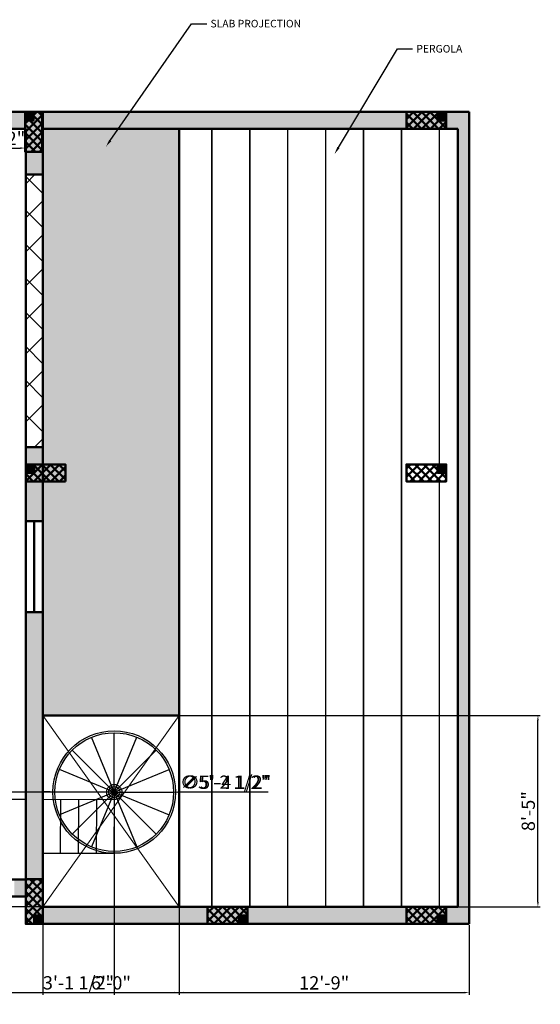
# Model space of a CAD drawing. Units: inches. Extents: x 1749 to 3550, y 1117 to 2383.
# Tile 12 of 15: x 3154 to 3428, y 1200 to 1720. Entities that reach past the tile are written whole.
import ezdxf
from ezdxf import colors
from ezdxf.entities.mleader import LeaderData, LeaderLine
from ezdxf.math import Vec2, Vec3

# ---------------------------------------------------------------- set-up
doc = ezdxf.new("R2010")
doc.units = ezdxf.units.IN
for name, color, linetype, lineweight in [('A-ANNO-DIMS', 2, 'Continuous', 18), ('A-ANNO-SYMB', 1, 'Continuous', 18), ('A-ANNO-TEXT', 3, 'Continuous', 18), ('A-COLS', 10, 'Continuous', 50), ('A-FLOR-STRS', 53, 'Continuous', 25), ('A-WALL', 7, 'Continuous', 50), ('A-WALL-PATT', 8, 'Continuous', 13)]:
    doc.layers.add(name, color=color, linetype=linetype, lineweight=lineweight)
doc.styles.get("Standard").update_dxf_attribs({"font": 'arial.ttf'})
doc.dimstyles.new('ISO-25', dxfattribs={"dimtxt": 7, "dimasz": 2.5, "dimexe": 1.25, "dimexo": 0.625, "dimtad": 1, "dimdec": 1, "dimlunit": 3, "dimtxsty": 'Standard', "dimcen": 2.5, "dimadec": 0, "dimazin": 0, "dimtfac": 1, "dimtdec": 1, "dimtmove": 0, "dimatfit": 3, "dimfxl": 1, "dimarcsym": 0})

# ---------------------------------------------------------------- blocks, each defined once
blk = doc.blocks.new('*D106')
at = {"layer": 'A-ANNO-DIMS', "color": 0, "lineweight": -2, "ltscale": 0.5, "transparency": 16777216}
for p, q in [((3122.34, 1661.76), (3122.34, 1651.06)), ((3156.55, 1661.76), (3156.55, 1651.06)), ((3124.84, 1652.31), (3154.05, 1652.31))]:
    blk.add_line(p, q, dxfattribs=at)
at = {"layer": 'A-ANNO-DIMS', "color": 0, "ltscale": 0.5, "transparency": 16777216}
for points in [[(3124.84, 1652.72), (3124.84, 1651.89), (3122.34, 1652.31)], [(3154.05, 1652.72), (3154.05, 1651.89), (3156.55, 1652.31)]]:
    blk.add_solid(points, dxfattribs=at)
at = {"layer": 'Defpoints', "color": 0, "ltscale": 0.5, "transparency": 16777216}
for p in [(3122.34, 1662.39), (3156.55, 1662.39), (3156.55, 1652.31)]:
    blk.add_point(p, dxfattribs=at)
at = {"layer": 'A-ANNO-DIMS', "color": 0, "ltscale": 0.5, "transparency": 16777216, "insert": (3139.44, 1656.51), "char_height": 7, "attachment_point": 5}
blk.add_mtext('2\'-10.2"', dxfattribs=at)
blk = doc.blocks.new('*D199')
at = {"layer": 'A-ANNO-DIMS', "color": 0, "lineweight": -2, "ltscale": 0.5, "transparency": 16777216}
for p, q in [((2730.84, 1242.26), (2730.84, 1205.39)), ((3390.84, 1242.26), (3390.84, 1205.39)), ((2733.34, 1206.64), (3388.34, 1206.64))]:
    blk.add_line(p, q, dxfattribs=at)
at = {"layer": 'A-ANNO-DIMS', "color": 0, "ltscale": 0.5, "transparency": 16777216}
for points in [[(2733.34, 1207.05), (2733.34, 1206.22), (2730.84, 1206.64)], [(3388.34, 1207.05), (3388.34, 1206.22), (3390.84, 1206.64)]]:
    blk.add_solid(points, dxfattribs=at)
at = {"layer": 'Defpoints', "color": 0, "ltscale": 0.5, "transparency": 16777216}
for p in [(2730.84, 1242.89), (3390.84, 1242.89), (3390.84, 1206.64)]:
    blk.add_point(p, dxfattribs=at)
at = {"layer": 'A-ANNO-DIMS', "color": 0, "ltscale": 0.5, "transparency": 16777216, "insert": (3060.84, 1210.84), "char_height": 7, "attachment_point": 5}
blk.add_mtext('55\'-0"', dxfattribs=at)
blk = doc.blocks.new('*D201')
at = {"layer": 'A-ANNO-DIMS', "color": 0, "lineweight": -2, "ltscale": 0.5, "transparency": 16777216}
for p, q in [((3237.84, 1251.26), (3237.84, 1205.39)), ((3165.84, 1242.26), (3165.84, 1205.39)), ((3168.34, 1206.64), (3235.34, 1206.64))]:
    blk.add_line(p, q, dxfattribs=at)
at = {"layer": 'A-ANNO-DIMS', "color": 0, "ltscale": 0.5, "transparency": 16777216}
for points in [[(3168.34, 1207.05), (3168.34, 1206.22), (3165.84, 1206.64)], [(3235.34, 1207.05), (3235.34, 1206.22), (3237.84, 1206.64)]]:
    blk.add_solid(points, dxfattribs=at)
at = {"layer": 'Defpoints', "color": 0, "ltscale": 0.5, "transparency": 16777216}
for p in [(3237.84, 1251.89), (3165.84, 1242.89), (3237.84, 1206.64)]:
    blk.add_point(p, dxfattribs=at)
at = {"layer": 'A-ANNO-DIMS', "color": 0, "ltscale": 0.5, "transparency": 16777216, "insert": (3201.84, 1210.84), "char_height": 7, "attachment_point": 5}
blk.add_mtext('6\'-0"', dxfattribs=at)
blk = doc.blocks.new('*D202')
at = {"layer": 'A-ANNO-DIMS', "color": 0, "lineweight": -2, "ltscale": 0.5, "transparency": 16777216}
for p, q in [((3237.84, 1251.26), (3237.84, 1205.39)), ((3390.84, 1242.26), (3390.84, 1205.39)), ((3240.34, 1206.64), (3388.34, 1206.64))]:
    blk.add_line(p, q, dxfattribs=at)
at = {"layer": 'A-ANNO-DIMS', "color": 0, "ltscale": 0.5, "transparency": 16777216}
for points in [[(3240.34, 1207.05), (3240.34, 1206.22), (3237.84, 1206.64)], [(3388.34, 1207.05), (3388.34, 1206.22), (3390.84, 1206.64)]]:
    blk.add_solid(points, dxfattribs=at)
at = {"layer": 'Defpoints', "color": 0, "ltscale": 0.5, "transparency": 16777216}
for p in [(3237.84, 1251.89), (3390.84, 1242.89), (3390.84, 1206.64)]:
    blk.add_point(p, dxfattribs=at)
at = {"layer": 'A-ANNO-DIMS', "color": 0, "ltscale": 0.5, "transparency": 16777216, "insert": (3314.34, 1210.84), "char_height": 7, "attachment_point": 5}
blk.add_mtext('12\'-9"', dxfattribs=at)
blk = doc.blocks.new('*D203')
at = {"layer": 'A-ANNO-DIMS', "color": 0, "lineweight": -2, "ltscale": 0.5, "transparency": 16777216}
for p, q in [((3203.57, 1311.82), (3203.57, 1205.39)), ((3165.84, 1308.09), (3165.84, 1205.39)), ((3168.34, 1206.64), (3201.07, 1206.64))]:
    blk.add_line(p, q, dxfattribs=at)
at = {"layer": 'A-ANNO-DIMS', "color": 0, "ltscale": 0.5, "transparency": 16777216}
for points in [[(3168.34, 1207.05), (3168.34, 1206.22), (3165.84, 1206.64)], [(3201.07, 1207.05), (3201.07, 1206.22), (3203.57, 1206.64)]]:
    blk.add_solid(points, dxfattribs=at)
at = {"layer": 'Defpoints', "color": 0, "ltscale": 0.5, "transparency": 16777216}
for p in [(3203.57, 1312.45), (3165.84, 1308.72), (3203.57, 1206.64)]:
    blk.add_point(p, dxfattribs=at)
at = {"layer": 'A-ANNO-DIMS', "color": 0, "ltscale": 0.5, "transparency": 16777216, "insert": (3184.7, 1210.88), "char_height": 7, "attachment_point": 5}
blk.add_mtext('3\'-1 1/2"', dxfattribs=at)
blk = doc.blocks.new('*D204')
at = {"layer": 'A-ANNO-DIMS', "color": 0, "lineweight": -2, "ltscale": 0.5, "transparency": 16777216}
for p, q in [((3202.94, 1312.45), (2693.34, 1312.45)), ((2694.59, 1254.39), (2694.59, 1309.95)), ((3165.21, 1251.89), (2693.34, 1251.89))]:
    blk.add_line(p, q, dxfattribs=at)
at = {"layer": 'A-ANNO-DIMS', "color": 0, "ltscale": 0.5, "transparency": 16777216}
for points in [[(2694.17, 1309.95), (2695, 1309.95), (2694.59, 1312.45)], [(2694.17, 1254.39), (2695, 1254.39), (2694.59, 1251.89)]]:
    blk.add_solid(points, dxfattribs=at)
at = {"layer": 'Defpoints', "color": 0, "ltscale": 0.5, "transparency": 16777216}
for p in [(2694.59, 1312.45), (3203.57, 1312.45), (3165.84, 1251.89)]:
    blk.add_point(p, dxfattribs=at)
at = {"layer": 'A-ANNO-DIMS', "color": 0, "ltscale": 0.5, "transparency": 16777216, "insert": (2690.34, 1282.17), "char_height": 7, "attachment_point": 5, "rotation": 90}
blk.add_mtext('5\'-0 1/2"', dxfattribs=at)
blk = doc.blocks.new('*D205')
at = {"layer": 'A-ANNO-DIMS', "color": 0, "lineweight": -2, "ltscale": 0.5, "transparency": 16777216}
for p, q in [((3238.46, 1352.89), (3428.34, 1352.89)), ((3427.09, 1254.39), (3427.09, 1350.39)), ((3238.46, 1251.89), (3428.34, 1251.89))]:
    blk.add_line(p, q, dxfattribs=at)
at = {"layer": 'A-ANNO-DIMS', "color": 0, "ltscale": 0.5, "transparency": 16777216}
for points in [[(3426.67, 1350.39), (3427.5, 1350.39), (3427.09, 1352.89)], [(3426.67, 1254.39), (3427.5, 1254.39), (3427.09, 1251.89)]]:
    blk.add_solid(points, dxfattribs=at)
at = {"layer": 'Defpoints', "color": 0, "ltscale": 0.5, "transparency": 16777216}
for p in [(3237.84, 1352.89), (3427.09, 1352.89), (3237.84, 1251.89)]:
    blk.add_point(p, dxfattribs=at)
at = {"layer": 'A-ANNO-DIMS', "color": 0, "ltscale": 0.5, "transparency": 16777216, "insert": (3422.89, 1302.39), "char_height": 7, "attachment_point": 5, "rotation": 90}
blk.add_mtext('8\'-5"', dxfattribs=at)
blk = doc.blocks.new('*D206')
at = {"layer": 'A-ANNO-DIMS', "color": 0, "lineweight": -2, "ltscale": 0.5, "transparency": 16777216}
for p, q in [((3168.73, 1312.5), (3166.23, 1312.5)), ((3171.23, 1312.49), (3235.9, 1312.4)), ((3284.69, 1312.33), (3238.4, 1312.4))]:
    blk.add_line(p, q, dxfattribs=at)
at = {"layer": 'A-ANNO-DIMS', "color": 0, "ltscale": 0.5, "transparency": 16777216}
for points in [[(3168.73, 1312.91), (3168.73, 1312.08), (3171.23, 1312.49)], [(3238.4, 1312.81), (3238.4, 1311.98), (3235.9, 1312.4)]]:
    blk.add_solid(points, dxfattribs=at)
at = {"layer": 'Defpoints', "color": 0, "ltscale": 0.5, "transparency": 16777216}
for p in [(3171.23, 1312.49), (3235.9, 1312.4)]:
    blk.add_point(p, dxfattribs=at)
at = {"layer": 'A-ANNO-DIMS', "color": 0, "ltscale": 0.5, "transparency": 16777216, "insert": (3262.8, 1316.76), "char_height": 7, "attachment_point": 5, "rotation": 359.9168}
blk.add_mtext('∅5\'-4 1/2"', dxfattribs=at)
blk = doc.blocks.new('*D207')
at = {"layer": 'A-ANNO-DIMS', "color": 0, "lineweight": -2, "ltscale": 0.5, "transparency": 16777216}
for p, q in [((3169.73, 1312.5), (3167.23, 1312.5)), ((3172.23, 1312.49), (3234.9, 1312.4)), ((3283.69, 1312.33), (3237.4, 1312.4))]:
    blk.add_line(p, q, dxfattribs=at)
at = {"layer": 'A-ANNO-DIMS', "color": 0, "ltscale": 0.5, "transparency": 16777216}
for points in [[(3169.73, 1312.91), (3169.73, 1312.08), (3172.23, 1312.49)], [(3237.4, 1312.81), (3237.4, 1311.98), (3234.9, 1312.4)]]:
    blk.add_solid(points, dxfattribs=at)
at = {"layer": 'Defpoints', "color": 0, "ltscale": 0.5, "transparency": 16777216}
for p in [(3172.23, 1312.49), (3234.9, 1312.4)]:
    blk.add_point(p, dxfattribs=at)
at = {"layer": 'A-ANNO-DIMS', "color": 0, "ltscale": 0.5, "transparency": 16777216, "insert": (3261.8, 1316.75), "char_height": 7, "attachment_point": 5, "rotation": 359.9141}
blk.add_mtext('∅5\'-2 1/2"', dxfattribs=at)

msp = doc.modelspace()

# ---------------------------------------------------------------- hatches: boundary and pattern name
at = {"layer": 'A-COLS', "ltscale": 10}
h = msp.add_hatch(color=256, dxfattribs=at)
h.dxf.hatch_style = 1
h.paths.add_polyline_path([(3156.55, 1671.39), (3156.55, 1666.89), (3161.05, 1666.89), (3161.05, 1671.39)])
h = msp.add_hatch(dxfattribs=at)
h.set_pattern_fill('ANSI37', color=256, angle=90)
h.set_pattern_definition([(135, (4539.2875, -0.8568), (-2.245064, -2.245064), []), (225, (4539.2875, -0.8568), (2.245064, -2.245064), [])])
h.paths.add_polyline_path([(3156.55, 1650.39), (3165.55, 1650.39), (3165.55, 1671.39), (3156.55, 1671.39)])
h = msp.add_hatch(dxfattribs=at)
h.set_pattern_fill('ANSI37', color=256, angle=180)
h.set_pattern_definition([(225, (5065.2954, 3029.4936), (2.245064, -2.245064), []), (315, (5065.2954, 3029.4936), (2.245064, 2.245064), [])])
h.paths.add_polyline_path([(3357.68, 1671.39), (3357.68, 1662.39), (3378.68, 1662.39), (3378.68, 1671.39)])
h = msp.add_hatch(color=256, dxfattribs=at)
h.dxf.hatch_style = 1
h.paths.add_polyline_path([(3378.68, 1671.39), (3374.18, 1671.39), (3374.18, 1666.89), (3378.68, 1666.89)])
h = msp.add_hatch(color=256, dxfattribs=at)
h.dxf.hatch_style = 1
h.paths.add_polyline_path([(3156.84, 1480.89), (3161.34, 1480.89), (3161.34, 1485.39), (3156.84, 1485.39)])
h = msp.add_hatch(dxfattribs=at)
h.set_pattern_fill('ANSI37', color=256, angle=180)
h.set_pattern_definition([(225, (4829.08, 2843.4936), (2.245064, -2.245064), []), (315, (4829.08, 2843.4936), (2.245064, 2.245064), [])])
h.paths.add_polyline_path([(3156.84, 1485.39), (3156.84, 1476.39), (3177.84, 1476.39), (3177.84, 1485.39)])
h = msp.add_hatch(dxfattribs=at)
h.set_pattern_fill('ANSI37', color=256, angle=360)
h.set_pattern_definition([(45, (1706.44, 96.9624), (-2.245064, 2.245064), []), (135, (1706.44, 96.9624), (-2.245064, -2.245064), [])])
h.paths.add_polyline_path([(3357.68, 1485.39), (3357.68, 1476.39), (3378.68, 1476.39), (3378.68, 1485.39)])
h = msp.add_hatch(color=256, dxfattribs=at)
h.dxf.hatch_style = 1
h.paths.add_polyline_path([(3378.68, 1485.39), (3374.18, 1485.39), (3374.18, 1480.89), (3378.68, 1480.89)])
h = msp.add_hatch(dxfattribs=at)
h.set_pattern_fill('ANSI37', color=256, angle=270)
h.set_pattern_definition([(315, (1770.86, 2915.132), (2.245064, 2.245064), []), (45, (1770.86, 2915.132), (-2.245064, 2.245064), [])])
h.paths.add_polyline_path([(3165.84, 1266.5), (3156.84, 1266.5), (3156.84, 1242.89), (3165.84, 1242.89)])
h = msp.add_hatch(color=256, dxfattribs=at)
h.dxf.hatch_style = 1
h.paths.add_polyline_path([(3165.84, 1242.89), (3165.84, 1247.39), (3161.34, 1247.39), (3161.34, 1242.89)])
h = msp.add_hatch(dxfattribs=at)
h.set_pattern_fill('ANSI37', color=256, angle=360)
h.set_pattern_definition([(45, (1601.591, -115.2184), (-2.245064, 2.245064), []), (135, (1601.591, -115.2184), (-2.245064, -2.245064), [])])
h.paths.add_polyline_path([(3273.84, 1242.89), (3273.84, 1251.89), (3252.84, 1251.89), (3252.84, 1242.89)])
h = msp.add_hatch(color=256, dxfattribs=at)
h.dxf.hatch_style = 1
h.paths.add_polyline_path([(3273.84, 1247.39), (3269.34, 1247.39), (3269.34, 1242.89), (3273.84, 1242.89)])
h = msp.add_hatch(dxfattribs=at)
h.set_pattern_fill('ANSI37', color=256, angle=360)
h.set_pattern_definition([(45, (1706.44, -115.2184), (-2.245064, 2.245064), []), (135, (1706.44, -115.2184), (-2.245064, -2.245064), [])])
h.paths.add_polyline_path([(3378.68, 1242.89), (3378.68, 1251.89), (3357.68, 1251.89), (3357.68, 1242.89)])
h = msp.add_hatch(color=256, dxfattribs=at)
h.dxf.hatch_style = 1
h.paths.add_polyline_path([(3378.68, 1247.39), (3374.18, 1247.39), (3374.18, 1242.89), (3378.68, 1242.89)])
at = {"layer": 'A-WALL-PATT', "ltscale": 0.5}
h = msp.add_hatch(color=256, dxfattribs=at)
h.dxf.hatch_style = 1
h.paths.add_polyline_path([(3156.84, 1662.39), (3156.84, 1638.39), (3165.84, 1638.39), (3165.84, 1662.39), (3165.84, 1671.39), (3122.34, 1671.39), (3122.34, 1662.39)])
h = msp.add_hatch(color=256, dxfattribs=at)
h.dxf.hatch_style = 1
h.paths.add_polyline_path([(3165.84, 1671.39), (3165.84, 1662.39), (3384.84, 1662.39), (3384.84, 1251.89), (3165.84, 1251.89), (3165.84, 1242.89), (3390.84, 1242.89), (3390.84, 1671.39)])
h = msp.add_hatch(color=256, dxfattribs=at)
h.dxf.hatch_style = 1
h.paths.add_polyline_path([(3237.84, 1662.39), (3165.84, 1662.39), (3165.84, 1352.89), (3237.84, 1352.89)])
h = msp.add_hatch(dxfattribs=at)
h.set_pattern_fill('JIS_LC_20', color=256, angle=45)
h.set_pattern_definition([(90, (1254.935, 1815.002), (-20, 0), []), (90, (1255.218, 1815.285), (-20, 0), [])])
h.paths.add_polyline_path([(3237.84, 1352.89), (3237.84, 1251.89), (3384.84, 1251.89), (3384.84, 1662.39), (3237.84, 1662.39)])
h.paths.add_polyline_path([(3357.68, 1485.39), (3378.68, 1485.39), (3378.68, 1476.39), (3357.68, 1476.39)], flags=16)
h.paths.add_polyline_path([(3374.18, 1485.39), (3378.68, 1485.39), (3378.68, 1480.89), (3374.18, 1480.89)], flags=0)
h = msp.add_hatch(dxfattribs=at)
h.set_pattern_fill('ANSI37', color=256, scale=4)
h.set_pattern_definition([(45, (1254.935, 1815.002), (-8.98026, 8.98026), []), (135, (1254.935, 1815.002), (-8.98026, -8.98026), [])])
h.paths.add_polyline_path([(3156.84, 1494.39), (3165.84, 1494.39), (3165.84, 1638.39), (3156.84, 1638.39)])
h = msp.add_hatch(color=256, dxfattribs=at)
h.dxf.hatch_style = 1
h.paths.add_polyline_path([(3156.84, 1455.39), (3165.84, 1455.39), (3165.84, 1494.39), (3156.84, 1494.39), (3156.84, 1485.39), (3156.84, 1476.39)])
h = msp.add_hatch(color=256, dxfattribs=at)
h.dxf.hatch_style = 1
h.paths.add_polyline_path([(3156.84, 1266.39), (3150.84, 1266.39), (3150.84, 1257.39), (3156.84, 1257.39), (3156.84, 1242.89), (3165.84, 1242.89), (3165.84, 1251.89), (3165.84, 1407.39), (3156.84, 1407.39)])

# ---------------------------------------------------------------- linework, layer by layer
at = {"layer": 'A-ANNO-SYMB', "ltscale": 0.5}
for p, q in [((3237.84, 1352.89), (3165.84, 1251.89)), ((3165.84, 1352.89), (3237.84, 1251.89))]:
    msp.add_line(p, q, dxfattribs=at)
at = {"layer": 'A-COLS', "ltscale": 0.5}
for p, q in [((3156.84, 1494.39), (3156.84, 1485.39)), ((3156.84, 1485.39), (3165.84, 1485.39))]:
    msp.add_line(p, q, dxfattribs=at)
at = {"layer": 'A-COLS', "ltscale": 10}
for points in [[(3161.05, 1671.39), (3156.55, 1671.39), (3156.55, 1666.89), (3161.05, 1666.89)], [(3165.55, 1650.39), (3165.55, 1671.39), (3156.55, 1671.39), (3156.55, 1650.39)], [(3357.68, 1662.39), (3378.68, 1662.39), (3378.68, 1671.39), (3357.68, 1671.39)], [(3378.68, 1666.89), (3378.68, 1671.39), (3374.18, 1671.39), (3374.18, 1666.89)], [(3156.84, 1480.89), (3156.84, 1485.39), (3161.34, 1485.39), (3161.34, 1480.89)], [(3177.84, 1476.39), (3156.84, 1476.39), (3156.84, 1485.39), (3177.84, 1485.39)], [(3357.68, 1476.39), (3378.68, 1476.39), (3378.68, 1485.39), (3357.68, 1485.39)], [(3378.68, 1480.89), (3378.68, 1485.39), (3374.18, 1485.39), (3374.18, 1480.89)], [(3156.84, 1266.5), (3156.84, 1242.89), (3165.84, 1242.89), (3165.84, 1266.5)], [(3161.34, 1242.89), (3165.84, 1242.89), (3165.84, 1247.39), (3161.34, 1247.39)], [(3252.84, 1251.89), (3273.84, 1251.89), (3273.84, 1242.89), (3252.84, 1242.89)], [(3273.84, 1247.39), (3273.84, 1242.89), (3269.34, 1242.89), (3269.34, 1247.39)], [(3357.68, 1251.89), (3378.68, 1251.89), (3378.68, 1242.89), (3357.68, 1242.89)], [(3378.68, 1247.39), (3378.68, 1242.89), (3374.18, 1242.89), (3374.18, 1247.39)]]:
    msp.add_lwpolyline(points, close=True, dxfattribs=at)
at = {"layer": 'A-FLOR-STRS', "ltscale": 0.5}
for p, q in [((3203.57, 1312.45), (3191.58, 1341.4)), ((3203.57, 1312.45), (3203.57, 1343.78)), ((3203.57, 1312.45), (3215.56, 1341.4)), ((3203.57, 1312.45), (3181.41, 1334.6)), ((3203.57, 1312.45), (3225.73, 1334.6)), ((3203.57, 1312.45), (3174.62, 1324.44)), ((3203.57, 1312.45), (3232.52, 1324.44)), ((3009.84, 1309.64), (3156.84, 1308.64)), ((3203.57, 1312.45), (3172.23, 1312.45)), ((3203.57, 1312.45), (3174.62, 1300.46)), ((3203.57, 1312.45), (3181.41, 1290.29)), ((3203.57, 1312.45), (3191.58, 1283.5)), ((3203.57, 1312.45), (3234.9, 1312.45)), ((3203.57, 1312.45), (3203.57, 1281.11)), ((3203.57, 1312.45), (3215.56, 1283.5)), ((3203.57, 1312.45), (3225.73, 1290.29)), ((3203.57, 1312.45), (3232.52, 1300.46)), ((3165.84, 1308.72), (3203.77, 1308.45)), ((3175.27, 1280.11), (3175.47, 1308.65)), ((3184.7, 1280.11), (3184.91, 1308.58)), ((3194.14, 1280.11), (3194.34, 1308.51)), ((3203.57, 1280.11), (3203.77, 1308.45)), ((3203.57, 1280.11), (3165.84, 1280.11)), ((3165.84, 1266.5), (3165.99, 1272.49))]:
    msp.add_line(p, q, dxfattribs=at)
for radius in [32.33, 31.33, 4, 3]:
    msp.add_circle((3203.57, 1312.45), radius, dxfattribs=at)
at = {"layer": 'A-WALL', "ltscale": 0.5}
for p, q in [((2730.84, 1671.39), (3390.84, 1671.39)), ((3165.84, 1662.39), (3165.84, 1671.39)), ((3390.84, 1671.39), (3390.84, 1242.89)), ((2739.84, 1662.39), (3156.84, 1662.39)), ((3156.84, 1662.39), (3156.84, 1485.39)), ((3165.84, 1662.39), (3165.84, 1251.89)), ((3165.84, 1662.39), (3384.84, 1662.39)), ((3237.84, 1662.39), (3237.84, 1352.89)), ((3384.84, 1662.39), (3384.84, 1251.89)), ((3156.84, 1638.39), (3165.84, 1638.39)), ((3156.84, 1494.39), (3165.84, 1494.39)), ((3156.84, 1485.39), (3156.84, 1476.39)), ((3156.84, 1476.39), (3156.84, 1266.39)), ((3156.84, 1455.39), (3165.84, 1455.39)), ((3161.34, 1455.39), (3161.34, 1407.39)), ((3156.84, 1407.39), (3165.84, 1407.39)), ((3237.84, 1352.89), (3165.84, 1352.89)), ((3237.84, 1352.89), (3237.84, 1251.89)), ((2973.84, 1266.39), (3156.84, 1266.39)), ((2973.84, 1257.39), (3156.84, 1257.39)), ((3156.84, 1257.39), (3156.84, 1242.89)), ((3165.84, 1251.89), (3384.84, 1251.89)), ((3165.84, 1251.89), (3165.84, 1242.89)), ((3156.84, 1242.89), (3390.84, 1242.89))]:
    msp.add_line(p, q, dxfattribs=at)

# ---------------------------------------------------------------- dimensions: what is measured, and where the dimension line sits
at = {"layer": 'A-ANNO-DIMS', "ltscale": 0.5}
for base, p1, p2, override, picture, middle in [((3156.55, 1652.31), (3122.34, 1662.39), (3156.55, 1662.39), {"dimclrd": 0, "dimclre": 0, "dimclrt": 0}, '*D106', (3139.44, 1656.51)), ((3203.57, 1206.64), (3165.84, 1308.72), (3203.57, 1312.45), {"dimdec": 1, "dimlfac": 1, "dimrnd": 0, "dimzin": 1, "dimdsep": 46, "dimlunit": 4, "dimfrac": 2}, '*D203', (3184.7, 1210.88)), ((3237.84, 1206.64), (3165.84, 1242.89), (3237.84, 1251.89), {"dimdec": 1, "dimlfac": 1, "dimrnd": 0, "dimzin": 1, "dimdsep": 46, "dimlunit": 4, "dimfrac": 2}, '*D201', (3201.84, 1210.84)), ((3390.84, 1206.64), (3237.84, 1251.89), (3390.84, 1242.89), {"dimdec": 1, "dimlfac": 1, "dimrnd": 0, "dimzin": 1, "dimdsep": 46, "dimlunit": 4, "dimfrac": 2}, '*D202', (3314.34, 1210.84)), ((3390.84, 1206.64), (2730.84, 1242.89), (3390.84, 1242.89), {"dimdec": 1, "dimlfac": 1, "dimrnd": 0, "dimzin": 1, "dimdsep": 46, "dimlunit": 4, "dimfrac": 2}, '*D199', (3060.84, 1210.84))]:
    dim = msp.add_linear_dim(base=base, p1=p1, p2=p2, dimstyle='ISO-25', override=override, dxfattribs=at)
    dim.commit()
    dim.dimension.update_dxf_attribs({"geometry": picture, "text_midpoint": middle})
for base, p1, p2, picture, middle in [((3427.09, 1352.89), (3237.84, 1251.89), (3237.84, 1352.89), '*D205', (3422.89, 1302.39)), ((2694.59, 1312.45), (3165.84, 1251.89), (3203.57, 1312.45), '*D204', (2690.34, 1282.17))]:
    dim = msp.add_linear_dim(base=base, p1=p1, p2=p2, angle=90, dimstyle='ISO-25', override={"dimdec": 1, "dimlfac": 1, "dimrnd": 0, "dimzin": 1, "dimdsep": 46, "dimlunit": 4, "dimfrac": 2}, dxfattribs=at)
    dim.commit()
    dim.dimension.update_dxf_attribs({"geometry": picture, "text_midpoint": middle})
dim = msp.add_diameter_dim_2p(p1=(3171.23, 1312.49), p2=(3235.9, 1312.4), dimstyle='ISO-25', override={"dimdec": 1, "dimlfac": 1, "dimrnd": 0, "dimzin": 1, "dimdsep": 46, "dimlunit": 4, "dimfrac": 2}, dxfattribs=at)
dim.commit()
dim.dimension.update_dxf_attribs({"geometry": '*D206', "text_midpoint": (3262.8, 1312.36)})
dim = msp.add_diameter_dim_2p(p1=(3172.23, 1312.49), p2=(3234.9, 1312.4), dimstyle='ISO-25', override={"dimdec": 1, "dimlfac": 1, "dimrnd": 0, "dimzin": 1, "dimdsep": 46, "dimlunit": 4, "dimfrac": 2}, dxfattribs=at)
dim.commit()
dim.dimension.update_dxf_attribs({"geometry": '*D207', "text_midpoint": (3261.8, 1312.36), "dimtype": 163})

# ---------------------------------------------------------------- leaders
at = {"layer": 'A-ANNO-TEXT', "ltscale": 0.5}
ml = msp.add_multileader_mtext('Standard', dxfattribs=at)
ml.set_content('SLAB PROJECTION', color=256)
ml.set_leader_properties()
ml.build(insert=Vec2(0, 0))
ctx = ml.context
ctx.base_point, ctx.plane_origin = Vec3(3252.35, 1717.94), Vec3(3199.19, 1653)
notes = []
notes.append((ctx, [(0, (1, 1, 0), (3244.35, 1717.94), (1, 0), 8, [(0, [(3199.19, 1653)], 0, [])])]))
ctx.mtext.insert, ctx.mtext.flow_direction = Vec3(3254.35, 1719.98), 5
ml = msp.add_multileader_mtext('Standard', dxfattribs=at)
ml.set_content('PERGOLA', color=256)
ml.set_leader_properties()
ml.build(insert=Vec2(0, 0))
ctx = ml.context
ctx.base_point, ctx.plane_origin = Vec3(3360.96, 1704.67), Vec3(3319.79, 1649.15)
notes.append((ctx, [(0, (1, 1, 0), (3352.96, 1704.67), (1, 0), 8, [(0, [(3319.79, 1649.15)], 0, [])])]))
ctx.mtext.insert, ctx.mtext.flow_direction = Vec3(3362.96, 1706.71), 5
for ctx, leaders in notes:
    for number, flags, end, landing, length, lines in leaders:
        leader = LeaderData()
        leader.index, (leader.has_last_leader_line, leader.has_dogleg_vector, leader.attachment_direction) = number, flags
        leader.last_leader_point, leader.dogleg_vector, leader.dogleg_length = Vec3(end), Vec3(landing), length
        for number, points, colour, breaks in lines:
            line = LeaderLine()
            line.index, line.vertices, line.color, line.breaks = number, Vec3.list(points), colors.encode_raw_color(colour), breaks
            leader.lines.append(line)
        ctx.leaders.append(leader)

doc.saveas('drawing.dxf')
